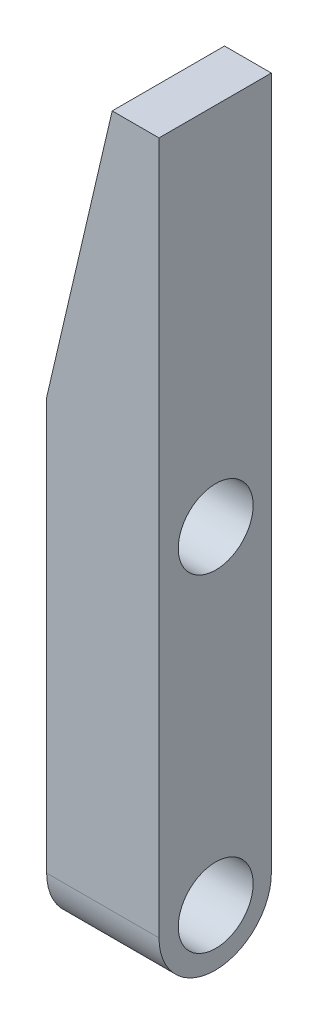
SolidWorks part; units mm, degrees
material "Plain Carbon Steel"
ref_plane "Front Plane" through (0, 0, 0) normal (0, 0, 1) x (1, 0, 0)
ref_plane "Top Plane" through (0, 0, 0) normal (0, 1, 0) x (1, 0, 0)
ref_plane "Right Plane" through (0, 0, 0) normal (1, 0, 0) x (0, 0, -1)
sketch "Jaw Profile Sketch" plane through (0, 0, 0) normal (0, 0, 1) x (1, 0, 0)
  line L0 (0, 0) -> (-5, 0)
  line L1 (-5, 0) -> (-12, -30)
  line L2 (-12, -30) -> (-12, -74)
  line L3 (-12, -74) -> (0, -74)
  line L4 (0, -74) -> (0, 0)
  dimension "D1" = 5
  dimension "D2" = 30
  dimension "D3" = 12
  dimension "D4" = 74
extrude "Jaw Plate 12mm" add sketch "Jaw Profile Sketch" along normal mid plane 12
sketch "Rounded End Sketch" plane through (0, 0, 0) normal (1, 0, 0) x (0, 0, -1)
  line L0 (-6, -74) -> (6, -74) construction
  circle A0 centre (0, -74) radius 6
extrude "Rounded End Boss" add sketch "Rounded End Sketch" against normal up to surface (12 mm away) up to face at (-12, -52, 0)
hole_wizard "Tapped Hole M8x1.25" positions "3DSketch1" profile "Sketch6" tap size "M8x1.25" standard "ANSI Metric" end condition up to next
sketch3d "3DSketch1"
  point P0 (0, -74, -0.0558)
  point P2 (0, -39, -0.0558)
  dimension "D1" = 35
sketch "Sketch6" plane through (0, -74, -0.0558) normal (0, 1, 0) x (0, 0, -1)
  line L0 (0, 0) -> (0, 12)
  line L1 (0, 12) -> (4, 12)
  line L2 (4, 12) -> (4, 0)
  line L5 (4, 0) -> (0, 0)
  line L11 (0, -6.35) -> (0, 107.95) construction
  dimension "Thread Major Dia." = 8
  dimension "Thru Tap Drill Depth" = 12
